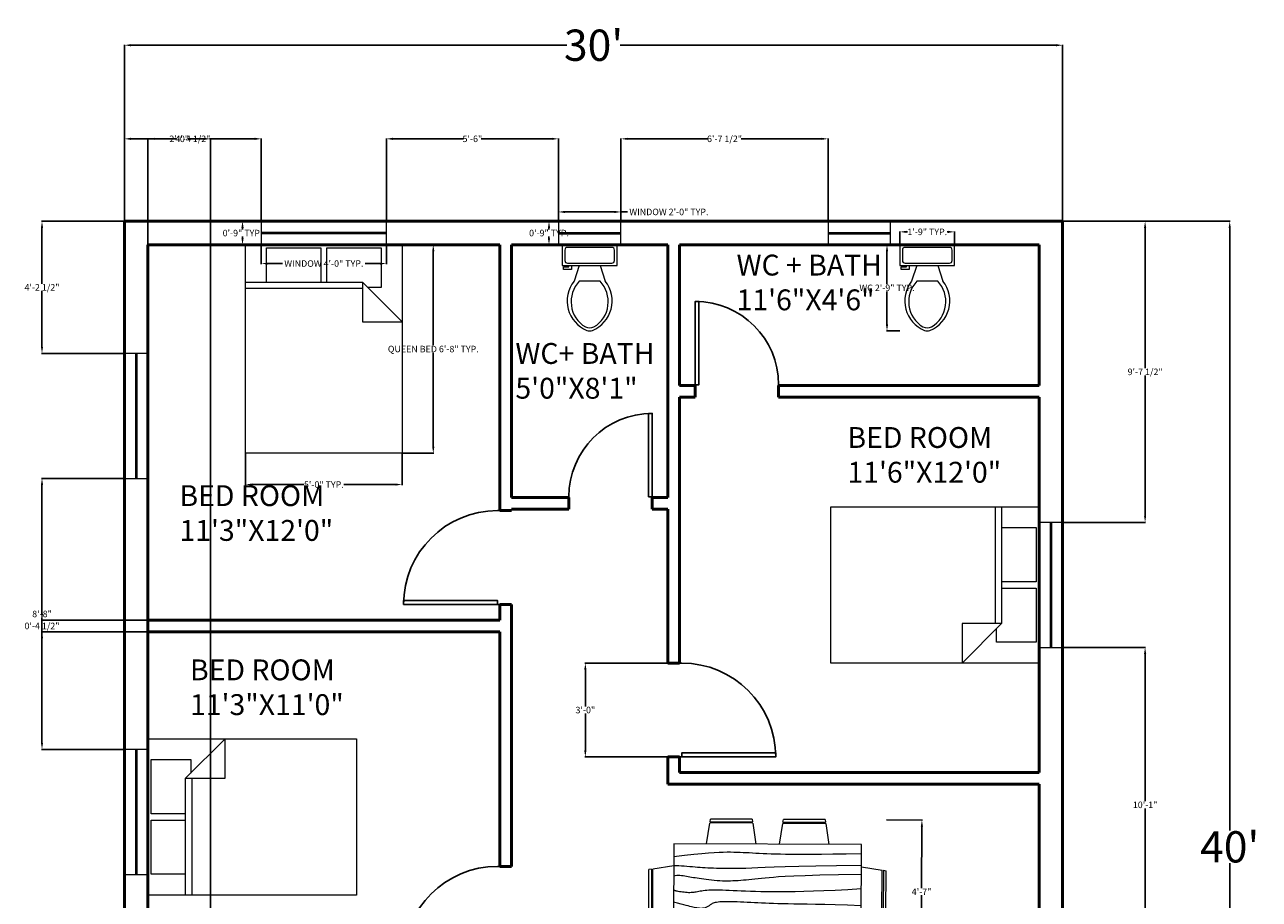
# Model space of a CAD drawing. Units: inches. Extents: x 14 to 510, y 5 to 635.
# Tile 3 of 3: x 18 to 492, y 299 to 635. Entities that reach past the tile are written whole.
import ezdxf

# ---------------------------------------------------------------- set-up
doc = ezdxf.new("R2010")
doc.units = ezdxf.units.IN
doc.header["$MEASUREMENT"] = 0
for name, color, linetype, lineweight in [('A-ANNO-DIMS', 210, 'Continuous', 18), ('A-AREA-IDEN', 210, 'Continuous', 25), ('A-FLOR-FIXT', 100, 'Continuous', 18), ('A-FURN', 100, 'Continuous', 18), ('DOOR', 20, 'Continuous', 25), ('WALL', 40, 'Continuous', 50), ('WINDOW', 131, 'Continuous', 18)]:
    doc.layers.add(name, color=color, linetype=linetype, lineweight=lineweight)
doc.styles.get("Standard").update_dxf_attribs({"font": 'arial.ttf'})
doc.dimstyles.get("Standard").update_dxf_attribs({"dimtxt": 2.5, "dimasz": 2.5, "dimexe": 0.18, "dimexo": 0.0625, "dimgap": 0.09, "dimtad": 0, "dimtih": 1, "dimtoh": 1, "dimzin": 0, "dimdsep": 46, "dimlunit": 3, "dimtxsty": 'Standard', "dimcen": 0.09, "dimadec": 0, "dimazin": 0, "dimtfac": 1, "dimtofl": 0, "dimtmove": 0, "dimatfit": 3, "dimfxl": 1, "dimtolj": 1, "dimtzin": 0, "dimarcsym": 0})

# ---------------------------------------------------------------- blocks, each defined once
blk = doc.blocks.new('*U2')
for p, q in [((0, 0), (0, -6)), ((40, 0), (40, -6))]:
    blk.add_line(p, q)
blk.add_lwpolyline([(0, 0), (0, 40), (1.75, 40), (1.75, 0)], close=True)
blk.add_arc((0, 0), 40, 0, 90)
blk = doc.blocks.new('Dining Set - 36 x 72 in.')
for p, q in [((-22.2343, 26.00059), (-23.4847, 17.99762)), ((-22.2304, 26), (-5.7608, 26)), ((-22, 27.5), (-22.1562, 26.50042)), ((-5.8416, 26.5), (-22.1534, 26.5)), ((-22, 27.5), (-6, 27.5)), ((-5.8437, 26.49966), (-6, 27.5)), ((-4.5152, 17.99762), (-5.7655, 25.99926)), ((5.7657, 26.00059), (4.5153, 17.99762)), ((5.7696, 26), (22.2392, 26)), ((6, 27.5), (5.8438, 26.50042)), ((22.1584, 26.5), (5.8466, 26.5)), ((6, 27.5), (22, 27.5)), ((22.1563, 26.49966), (22, 27.5)), ((23.4848, 17.99762), (22.2345, 25.99926)), ((36, 18), (-36, 18)), ((-36, 18), (-36, -18)), ((36, -18), (36, 18)), ((-44.0006, 8.23428), (-35.9976, 9.48474)), ((44.0006, 8.23428), (35.9976, 9.48474)), ((-45.5, 8), (-44.5004, 8.15617)), ((-45.5, 8), (-45.5, -8)), ((-44.5, -8.15843), (-44.5, 8.15338)), ((-44, 8.23041), (-44, -8.23915)), ((44, 8.23041), (44, -8.23915)), ((44.5, -8.15843), (44.5, 8.15338)), ((45.5, 8), (44.5005, 8.15617)), ((45.5, 8), (45.5, -8)), ((-44.4997, -8.15631), (-45.5, -8)), ((-35.9976, -9.48476), (-43.9993, -8.2345)), ((35.9976, -9.48476), (43.9993, -8.2345)), ((44.4997, -8.15631), (45.5, -8)), ((-36, -18), (36, -18)), ((-22.2343, -26.0006), (-23.4847, -17.99762)), ((-4.5152, -17.99762), (-5.7655, -25.99928)), ((5.7657, -26.0006), (4.5153, -17.99762)), ((23.4848, -17.99762), (22.2345, -25.99928)), ((-22.2304, -26), (-5.7608, -26)), ((-22, -27.5), (-22.1562, -26.50044)), ((-5.8416, -26.5), (-22.1534, -26.5)), ((-22, -27.5), (-6, -27.5)), ((-5.8437, -26.49967), (-6, -27.5)), ((5.7696, -26), (22.2392, -26)), ((6, -27.5), (5.8438, -26.50044)), ((22.1584, -26.5), (5.8466, -26.5)), ((6, -27.5), (22, -27.5)), ((22.1563, -26.49967), (22, -27.5))]:
    blk.add_line(p, q)
for points in [[(-36, 15), (-31.1772, 14.97754), (-26.8079, 14.91406), (-22.8538, 14.81543), (-19.276, 14.6875), (-16.0362, 14.53613), (-13.0957, 14.36718), (-10.4159, 14.18652), (-7.9583, 14), (-5.6904, 13.81315), (-3.6035, 13.63021), (-1.6954, 13.45508), (0.0365, 13.29166), (1.5945, 13.14388), (2.9811, 13.01562), (4.1988, 12.9108), (5.25, 12.83333), (6.1393, 12.78613), (6.8802, 12.76823), (7.4883, 12.77767), (7.9792, 12.8125), (8.3685, 12.87077), (8.6719, 12.95052), (8.9049, 13.0498), (9.0833, 13.16666), (9.2205, 13.29899), (9.3216, 13.44401), (9.3895, 13.59879), (9.4271, 13.76041), (9.4373, 13.92594), (9.4232, 14.09245), (9.3875, 14.257), (9.3333, 14.41666), (9.2638, 14.56917), (9.1836, 14.71484), (9.0975, 14.85465), (9.0104, 14.98958), (8.9272, 15.1206), (8.8529, 15.2487), (8.7922, 15.37483), (8.75, 15.5), (8.7305, 15.62467), (8.7344, 15.74739), (8.7617, 15.86621), (8.8125, 15.97916), (8.8867, 16.08431), (8.9844, 16.17968), (9.1055, 16.26334), (9.25, 16.33333), (9.4189, 16.38802), (9.6172, 16.42708), (9.8506, 16.45052), (10.125, 16.45833), (10.4463, 16.45052), (10.8203, 16.42708), (11.2529, 16.38802), (11.75, 16.33333), (12.3184, 16.26318), (12.9694, 16.17838), (13.7151, 16.07991), (14.5677, 15.96875), (15.5395, 15.84586), (16.6426, 15.71224), (17.8893, 15.56884), (19.2917, 15.41666), (20.859, 15.25667), (22.5879, 15.08984), (24.4721, 14.91715), (26.5052, 14.73958), (28.6809, 14.5581), (30.9929, 14.3737), (33.4347, 14.18733), (36, 14)], [(-36, 10), (-28.9766, 10.14274), (-23.1725, 10.20442), (-18.4241, 10.19775), (-14.5677, 10.13541), (-11.4399, 10.03011), (-8.877, 9.89453), (-6.7154, 9.74137), (-4.7917, 9.58333), (-2.9698, 9.43082), (-1.2246, 9.28515), (0.4415, 9.14534), (2.026, 9.01041), (3.5266, 8.87939), (4.9408, 8.7513), (6.266, 8.62516), (7.5, 8.5), (8.6411, 8.37549), (9.6914, 8.2539), (10.6538, 8.13818), (11.5312, 8.03125), (12.3267, 7.93603), (13.043, 7.85547), (13.6831, 7.79248), (14.25, 7.75), (14.7471, 7.7303), (15.1797, 7.73307), (15.5537, 7.75732), (15.875, 7.80208), (16.1494, 7.86637), (16.3828, 7.94922), (16.5811, 8.04964), (16.75, 8.16666), (16.8944, 8.29915), (17.0143, 8.44531), (17.1089, 8.60319), (17.1771, 8.77083), (17.218, 8.94629), (17.2305, 9.1276), (17.2137, 9.31282), (17.1667, 9.5), (17.0895, 9.6875), (16.987, 9.875), (16.8649, 10.0625), (16.7292, 10.25), (16.5856, 10.4375), (16.4401, 10.625), (16.2985, 10.8125), (16.1667, 11), (16.05, 11.18733), (15.9518, 11.3737), (15.8752, 11.5581), (15.8229, 11.73958), (15.798, 11.91715), (15.8034, 12.08984), (15.842, 12.25667), (15.9167, 12.41666), (16.0295, 12.56836), (16.1784, 12.70833), (16.3605, 12.83268), (16.5729, 12.9375), (16.8127, 13.01888), (17.0768, 13.07291), (17.3625, 13.0957), (17.6667, 13.08333), (17.9894, 13.03312), (18.3418, 12.94726), (18.7382, 12.82918), (19.1927, 12.68229), (19.7195, 12.51001), (20.3327, 12.31575), (21.0465, 12.10294), (21.875, 11.875), (22.8357, 11.63354), (23.959, 11.37304), (25.2786, 11.08618), (26.8282, 10.76562), (28.6414, 10.40405), (30.752, 9.99414), (33.1936, 9.52856), (36, 9)], [(-36, 5.5), (-30.7157, 5.3348), (-26.069, 5.20963), (-21.9946, 5.11767), (-18.4271, 5.05208), (-15.3009, 5.00602), (-12.5508, 4.97265), (-10.1112, 4.94515), (-7.9167, 4.91666), (-5.909, 4.88167), (-4.0586, 4.83984), (-2.3429, 4.79215), (-0.7396, 4.73958), (0.7739, 4.6831), (2.22, 4.6237), (3.6213, 4.56233), (5, 4.5), (6.373, 4.43782), (7.7344, 4.3776), (9.0723, 4.32129), (10.375, 4.27083), (11.6309, 4.22819), (12.8281, 4.19531), (13.9551, 4.17415), (15, 4.16666), (15.954, 4.17448), (16.819, 4.19791), (17.6001, 4.23698), (18.3021, 4.29166), (18.9299, 4.36198), (19.4883, 4.44791), (19.9823, 4.54948), (20.4167, 4.66666), (20.7969, 4.79899), (21.1302, 4.94401), (21.4245, 5.09879), (21.6875, 5.26041), (21.9271, 5.42594), (22.1511, 5.59245), (22.3672, 5.757), (22.5834, 5.91666), (22.8065, 6.06868), (23.0404, 6.21093), (23.2879, 6.34147), (23.5521, 6.45833), (23.8358, 6.55957), (24.142, 6.64323), (24.4735, 6.70735), (24.8334, 6.75), (25.2235, 6.76969), (25.642, 6.76692), (26.0858, 6.74267), (26.5521, 6.69791), (27.0379, 6.63362), (27.5404, 6.55078), (28.0565, 6.45036), (28.5834, 6.33333), (29.1242, 6.19987), (29.7071, 6.04687), (30.3661, 5.87044), (31.1354, 5.66666), (32.0493, 5.43164), (33.142, 5.16146), (34.4475, 4.85221), (36, 4.5)], [(-36, -1), (-30.7915, -0.6591), (-26.0195, -0.38216), (-21.6519, -0.16284), (-17.6563, 0.00521), (-14.0005, 0.12833), (-10.6523, 0.21289), (-7.5796, 0.26522), (-4.75, 0.29166), (-2.134, 0.29793), (0.2878, 0.28711), (2.5317, 0.26163), (4.6146, 0.22396), (6.5529, 0.17651), (8.3633, 0.12174), (10.0623, 0.06209), (11.6667, 0), (13.1899, -0.06201), (14.6341, -0.1211), (15.9982, -0.17432), (17.2813, -0.21875), (18.4823, -0.25147), (19.6003, -0.26953), (20.6343, -0.27002), (21.5834, -0.25), (22.4481, -0.20768), (23.2357, -0.14584), (23.9549, -0.06836), (24.6146, 0.02083), (25.2235, 0.11784), (25.7904, 0.21875), (26.3241, 0.31966), (26.8334, 0.41666), (27.3265, 0.50618), (27.8099, 0.58593), (28.2894, 0.65397), (28.7709, 0.70833), (29.2601, 0.74707), (29.763, 0.76823), (30.2855, 0.76985), (30.8334, 0.75), (31.4088, 0.70784), (31.9994, 0.64713), (32.589, 0.57275), (33.1615, 0.48958), (33.7008, 0.4025), (34.1908, 0.3164), (34.6153, 0.23616), (34.9584, 0.16666), (35.2099, 0.11165), (35.3848, 0.07031), (35.504, 0.04069), (35.5886, 0.02083), (35.6594, 0.00879), (35.7377, 0.0026), (35.8442, 0.00032), (36, 0)], [(-36, -6.5), (-27.1843, -6.31267), (-20.084, -6.1263), (-14.469, -5.9419), (-10.1094, -5.76042), (-6.7752, -5.58285), (-4.2363, -5.41016), (-2.2629, -5.24333), (-0.625, -5.08334), (0.8708, -4.93099), (2.2715, -4.78646), (3.5872, -4.64974), (4.8281, -4.52084), (6.0046, -4.39974), (7.127, -4.28646), (8.2053, -4.18099), (9.25, -4.08334), (10.2705, -3.99382), (11.2734, -3.91407), (12.2647, -3.84603), (13.25, -3.79167), (14.2354, -3.75293), (15.2266, -3.73177), (16.2295, -3.73015), (17.25, -3.75), (18.2912, -3.79248), (19.3451, -3.85547), (20.4009, -3.93604), (21.4479, -4.03125), (22.4754, -4.13819), (23.4727, -4.25391), (24.4289, -4.37549), (25.3334, -4.5), (26.1785, -4.62492), (26.9694, -4.74935), (27.7145, -4.87281), (28.4219, -4.99479), (29.1, -5.11483), (29.7572, -5.23242), (30.4016, -5.34709), (31.0417, -5.45834), (31.6837, -5.56437), (32.3262, -5.65821), (32.9658, -5.73153), (33.599, -5.77604), (34.2224, -5.78345), (34.8327, -5.74545), (35.4264, -5.65373), (36, -5.5)], [(-36, -10), (-26.4022, -9.81299), (-18.4675, -9.62891), (-11.9839, -9.45069), (-6.7396, -9.28125), (-2.5226, -9.12354), (0.8789, -8.98047), (3.6769, -8.85498), (6.0833, -8.75), (8.2767, -8.66765), (10.3021, -8.60677), (12.1712, -8.56543), (13.8958, -8.54167), (15.4876, -8.53353), (16.9583, -8.53907), (18.3197, -8.55632), (19.5834, -8.58334), (20.7616, -8.61841), (21.8685, -8.66081), (22.9188, -8.71004), (23.9271, -8.76563), (24.9081, -8.82707), (25.8763, -8.89388), (26.8465, -8.96558), (27.8334, -9.04167), (28.8474, -9.12118), (29.8828, -9.20117), (30.93, -9.27824), (31.9792, -9.34896), (33.0205, -9.40991), (34.0443, -9.45768), (35.0407, -9.48885), (36, -9.5)], [(-36, -14.5), (-30.0881, -14.33513), (-25.0332, -14.21224), (-20.7312, -14.12647), (-17.0781, -14.07292), (-13.97, -14.04671), (-11.3027, -14.04297), (-8.9724, -14.05681), (-6.875, -14.08334), (-4.9224, -14.11833), (-3.0905, -14.16016), (-1.3709, -14.20785), (0.2448, -14.26042), (1.7647, -14.3169), (3.1973, -14.3763), (4.5507, -14.43767), (5.8333, -14.5), (7.0554, -14.5621), (8.235, -14.62175), (9.3922, -14.67652), (10.5469, -14.72396), (11.7192, -14.76164), (12.929, -14.78711), (14.1965, -14.79794), (15.5417, -14.79167), (16.9933, -14.76424), (18.6152, -14.70508), (20.4804, -14.60197), (22.6615, -14.44271), (25.2312, -14.21509), (28.2624, -13.9069), (31.8277, -13.50594), (36, -13)]]:
    blk.add_lwpolyline(points)
blk = doc.blocks.new('Bed - Queen')
for p, q in [((0, -80.00003), (0, 0)), ((0, 0), (59.99999, 0)), ((59.99999, 0), (59.99999, -80.00003)), ((7.99999, -1.2), (28.79998, -1.2)), ((7.99999, -14.4), (7.99999, -1.2)), ((28.79998, -1.2), (28.79998, -14.4)), ((31.19999, -1.2), (51.99999, -1.2)), ((31.19999, -14.4), (31.19999, -1.2)), ((51.99999, -1.2), (51.99999, -16.4)), ((0, -14.4), (44.8, -14.4)), ((44.8, -16.8), (0, -16.8)), ((59.99999, -29.6), (44.8, -14.4)), ((44.8, -14.4), (44.8, -29.6)), ((51.99999, -16.4), (46.79936, -16.4)), ((44.8, -29.6), (59.99999, -29.6)), ((59.99999, -80.00003), (0, -80.00003))]:
    blk.add_line(p, q)
blk = doc.blocks.new('Toilet - top')
for p, q in [((9.5, -6), (9.5, -2)), ((-10, -8.5), (-8, -8.5)), ((-10, -9.5), (-10, -8.5)), ((-8, -8.5), (-8, -8)), ((-7, -8), (-7, -9.5)), ((-4, -8), (-6, -14)), ((4, -8), (6, -14)), ((-7, -9.5), (-10, -9.5)), ((4, -14), (-4, -14))]:
    blk.add_line(p, q)
blk.add_lwpolyline([(10.5, -8), (10.5, 0), (-10.5, 0), (-10.5, -8)], close=True)
for points in [[(-9.5, -2), (-9.5, -6)], [(8.5, -1), (-8.5, -1)], [(-8.5, -7), (8.5, -7)]]:
    blk.add_lwpolyline(points)
for centre, radius, start, end in [((-8.62, -1.88), 0.884, 81.8699, 188.1301), ((8.62, -1.88), 0.884, 351.8699, 98.1301), ((-8.62, -6.12), 0.884, 171.8699, 278.1301), ((8.62, -6.12), 0.884, 261.8699, 8.1301), ((3.52, -21.58), 12.17, 141.4691, 247.9714), ((4.2, -21.82), 11.33, 136.3677, 238.9468), ((-3.52, -21.58), 12.17, 292.0284, 38.5307), ((-4.2, -21.82), 11.33, 301.053, 43.6321), ((0, -27.88), 4, 245.7318, 294.2682), ((0, -29), 4, 254.8605, 285.1395)]:
    blk.add_arc(centre, radius, start, end)
blk = doc.blocks.new('*D14')
at = {"layer": 'A-ANNO-DIMS', "color": 0, "lineweight": -2, "transparency": 16777216}
for p, q in [((416.67, 559.06), (480.9, 559.06)), ((480.72, 556.56), (480.72, 325.28)), ((480.72, 81.56), (480.72, 312.84)), ((416.67, 79.06), (480.9, 79.06))]:
    blk.add_line(p, q, dxfattribs=at)
at = {"layer": 'A-ANNO-DIMS', "color": 0, "transparency": 16777216}
for points in [[(480.3, 556.56), (481.13, 556.56), (480.72, 559.06)], [(480.3, 81.56), (481.13, 81.56), (480.72, 79.06)]]:
    blk.add_solid(points, dxfattribs=at)
at = {"layer": 'Defpoints', "color": 0, "transparency": 16777216}
for p in [(416.61, 559.06), (416.61, 79.06), (480.72, 79.06)]:
    blk.add_point(p, dxfattribs=at)
at = {"layer": 'A-ANNO-DIMS', "color": 0, "transparency": 16777216, "insert": (480.72, 319.06), "char_height": 12, "attachment_point": 5}
blk.add_mtext("\\A1;40'", dxfattribs=at)
blk = doc.blocks.new('*D15')
at = {"layer": 'A-ANNO-DIMS', "color": 0, "lineweight": -2, "transparency": 16777216}
for p, q in [((56.61, 559.12), (56.61, 626.81)), ((59.11, 626.63), (226.34, 626.63)), ((414.11, 626.63), (246.88, 626.63)), ((416.61, 559.12), (416.61, 626.81))]:
    blk.add_line(p, q, dxfattribs=at)
at = {"layer": 'A-ANNO-DIMS', "color": 0, "transparency": 16777216}
for points in [[(59.11, 627.05), (59.11, 626.21), (56.61, 626.63)], [(414.11, 627.05), (414.11, 626.21), (416.61, 626.63)]]:
    blk.add_solid(points, dxfattribs=at)
at = {"layer": 'Defpoints', "color": 0, "transparency": 16777216}
for p in [(416.61, 626.63), (56.61, 559.06), (416.61, 559.06)]:
    blk.add_point(p, dxfattribs=at)
at = {"layer": 'A-ANNO-DIMS', "color": 0, "transparency": 16777216, "insert": (236.61, 626.63), "char_height": 12, "attachment_point": 5}
blk.add_mtext("\\A1;30'", dxfattribs=at)
blk = doc.blocks.new('WIN-48IN')
for p, q in [((4.25, 48), (4.25, 0)), ((4.75, 48), (4.75, 0))]:
    blk.add_line(p, q)
blk.add_lwpolyline([(0, 48), (0, 0), (9, 0), (9, 48)], close=True)
blk = doc.blocks.new('WIN-24IN')
for p, q in [((0, 4.75), (24, 4.75)), ((0, 4.25), (24, 4.25))]:
    blk.add_line(p, q)
blk.add_lwpolyline([(0, 0), (24, 0), (24, 9), (0, 9)], close=True)
blk = doc.blocks.new('*D19')
at = {"layer": 'A-ANNO-DIMS', "color": 0, "lineweight": -2, "transparency": 16777216}
for p, q in [((109.11, 550), (109.11, 542.68)), ((157.11, 550), (157.11, 542.68)), ((111.61, 542.86), (117.2, 542.86)), ((154.61, 542.86), (149.02, 542.86))]:
    blk.add_line(p, q, dxfattribs=at)
at = {"layer": 'A-ANNO-DIMS', "color": 0, "transparency": 16777216}
for points in [[(111.61, 543.28), (111.61, 542.44), (109.11, 542.86)], [(154.61, 543.28), (154.61, 542.44), (157.11, 542.86)]]:
    blk.add_solid(points, dxfattribs=at)
at = {"layer": 'Defpoints', "color": 0, "transparency": 16777216}
for p in [(109.11, 550.06), (157.11, 550.06), (157.11, 542.86)]:
    blk.add_point(p, dxfattribs=at)
at = {"layer": 'A-ANNO-DIMS', "color": 0, "transparency": 16777216, "insert": (133.11, 542.86), "char_height": 2.5, "attachment_point": 5}
blk.add_mtext('\\A1;WINDOW 4\'-0" TYP.', dxfattribs=at)
blk = doc.blocks.new('*D20')
at = {"layer": 'A-ANNO-DIMS', "color": 0, "lineweight": -2, "transparency": 16777216}
for p, q in [((109.05, 559.06), (101.73, 559.06)), ((101.91, 556.56), (101.91, 555.93)), ((109.05, 550.06), (101.73, 550.06)), ((101.91, 552.56), (101.91, 553.19))]:
    blk.add_line(p, q, dxfattribs=at)
at = {"layer": 'A-ANNO-DIMS', "color": 0, "transparency": 16777216}
for points in [[(101.49, 556.56), (102.33, 556.56), (101.91, 559.06)], [(101.49, 552.56), (102.33, 552.56), (101.91, 550.06)]]:
    blk.add_solid(points, dxfattribs=at)
at = {"layer": 'Defpoints', "color": 0, "transparency": 16777216}
for p in [(109.11, 559.06), (101.91, 550.06), (109.11, 550.06)]:
    blk.add_point(p, dxfattribs=at)
at = {"layer": 'A-ANNO-DIMS', "color": 0, "transparency": 16777216, "insert": (101.91, 554.56), "char_height": 2.5, "attachment_point": 5}
blk.add_mtext('\\A1;0\'-9" TYP.', dxfattribs=at)
blk = doc.blocks.new('*D23')
at = {"layer": 'A-ANNO-DIMS', "color": 0, "lineweight": -2, "transparency": 16777216}
for p, q in [((223.11, 559.12), (223.11, 562.84)), ((225.61, 562.66), (244.61, 562.66)), ((247.11, 559.12), (247.11, 562.84)), ((247.11, 562.66), (249.61, 562.66))]:
    blk.add_line(p, q, dxfattribs=at)
at = {"layer": 'A-ANNO-DIMS', "color": 0, "transparency": 16777216}
for points in [[(225.61, 563.08), (225.61, 562.24), (223.11, 562.66)], [(244.61, 563.08), (244.61, 562.24), (247.11, 562.66)]]:
    blk.add_solid(points, dxfattribs=at)
at = {"layer": 'Defpoints', "color": 0, "transparency": 16777216}
for p in [(223.11, 559.06), (247.11, 562.66), (247.11, 559.06)]:
    blk.add_point(p, dxfattribs=at)
at = {"layer": 'A-ANNO-DIMS', "color": 0, "transparency": 16777216, "insert": (265.52, 562.66), "char_height": 2.5, "attachment_point": 5}
blk.add_mtext('\\A1;WINDOW 2\'-0" TYP.', dxfattribs=at)
blk = doc.blocks.new('*D24')
at = {"layer": 'A-ANNO-DIMS', "color": 0, "lineweight": -2, "transparency": 16777216}
for p, q in [((223.05, 559.06), (219.33, 559.06)), ((219.51, 556.56), (219.51, 555.93)), ((223.05, 550.06), (219.33, 550.06)), ((219.51, 552.56), (219.51, 553.19))]:
    blk.add_line(p, q, dxfattribs=at)
at = {"layer": 'A-ANNO-DIMS', "color": 0, "transparency": 16777216}
for points in [[(219.09, 556.56), (219.93, 556.56), (219.51, 559.06)], [(219.09, 552.56), (219.93, 552.56), (219.51, 550.06)]]:
    blk.add_solid(points, dxfattribs=at)
at = {"layer": 'Defpoints', "color": 0, "transparency": 16777216}
for p in [(219.51, 559.06), (223.11, 559.06), (223.11, 550.06)]:
    blk.add_point(p, dxfattribs=at)
at = {"layer": 'A-ANNO-DIMS', "color": 0, "transparency": 16777216, "insert": (219.51, 554.56), "char_height": 2.5, "attachment_point": 5}
blk.add_mtext('\\A1;0\'-9" TYP.', dxfattribs=at)
blk = doc.blocks.new('*D25')
at = {"layer": 'A-ANNO-DIMS', "color": 0, "lineweight": -2, "transparency": 16777216}
for p, q in [((163.17, 550.06), (175.29, 550.06)), ((175.11, 547.56), (175.11, 511.52)), ((175.11, 472.56), (175.11, 508.6)), ((163.17, 470.06), (175.29, 470.06))]:
    blk.add_line(p, q, dxfattribs=at)
at = {"layer": 'A-ANNO-DIMS', "color": 0, "transparency": 16777216}
for points in [[(174.69, 547.56), (175.53, 547.56), (175.11, 550.06)], [(174.69, 472.56), (175.53, 472.56), (175.11, 470.06)]]:
    blk.add_solid(points, dxfattribs=at)
at = {"layer": 'Defpoints', "color": 0, "transparency": 16777216}
for p in [(163.11, 550.06), (175.11, 550.06), (163.11, 470.06)]:
    blk.add_point(p, dxfattribs=at)
at = {"layer": 'A-ANNO-DIMS', "color": 0, "transparency": 16777216, "insert": (175.11, 510.06), "char_height": 2.5, "attachment_point": 5}
blk.add_mtext('\\A1;QUEEN BED 6\'-8" TYP.', dxfattribs=at)
blk = doc.blocks.new('*D26')
at = {"layer": 'A-ANNO-DIMS', "color": 0, "lineweight": -2, "transparency": 16777216}
for p, q in [((103.11, 470), (103.11, 457.88)), ((163.11, 470), (163.11, 457.88)), ((105.61, 458.06), (125.4, 458.06)), ((160.61, 458.06), (140.82, 458.06))]:
    blk.add_line(p, q, dxfattribs=at)
at = {"layer": 'A-ANNO-DIMS', "color": 0, "transparency": 16777216}
for points in [[(105.61, 458.48), (105.61, 457.64), (103.11, 458.06)], [(160.61, 458.48), (160.61, 457.64), (163.11, 458.06)]]:
    blk.add_solid(points, dxfattribs=at)
at = {"layer": 'Defpoints', "color": 0, "transparency": 16777216}
for p in [(103.11, 470.06), (163.11, 470.06), (163.11, 458.06)]:
    blk.add_point(p, dxfattribs=at)
at = {"layer": 'A-ANNO-DIMS', "color": 0, "transparency": 16777216, "insert": (133.11, 458.06), "char_height": 2.5, "attachment_point": 5}
blk.add_mtext('\\A1;5\'-0" TYP.', dxfattribs=at)
blk = doc.blocks.new('*D27')
at = {"layer": 'A-ANNO-DIMS', "color": 0, "lineweight": -2, "transparency": 16777216}
for p, q in [((354.1, 550.06), (349.03, 550.06)), ((349.21, 547.56), (349.21, 534.92)), ((349.21, 519.51), (349.21, 532.16)), ((354.1, 517.01), (349.03, 517.01))]:
    blk.add_line(p, q, dxfattribs=at)
at = {"layer": 'A-ANNO-DIMS', "color": 0, "transparency": 16777216}
for points in [[(348.79, 547.56), (349.63, 547.56), (349.21, 550.06)], [(348.79, 519.51), (349.63, 519.51), (349.21, 517.01)]]:
    blk.add_solid(points, dxfattribs=at)
at = {"layer": 'Defpoints', "color": 0, "transparency": 16777216}
for p in [(349.21, 550.06), (354.17, 550.06), (354.17, 517.01)]:
    blk.add_point(p, dxfattribs=at)
at = {"layer": 'A-ANNO-DIMS', "color": 0, "transparency": 16777216, "insert": (349.21, 533.54), "char_height": 2.5, "attachment_point": 5}
blk.add_mtext('\\A1;WC 2\'-9" TYP.', dxfattribs=at)
blk = doc.blocks.new('*D28')
at = {"layer": 'A-ANNO-DIMS', "color": 0, "lineweight": -2, "transparency": 16777216}
for p, q in [((354.17, 550.12), (354.17, 555.2)), ((356.67, 555.02), (357.07, 555.02)), ((372.67, 555.02), (372.26, 555.02)), ((375.17, 550.12), (375.17, 555.2))]:
    blk.add_line(p, q, dxfattribs=at)
at = {"layer": 'A-ANNO-DIMS', "color": 0, "transparency": 16777216}
for points in [[(356.67, 555.43), (356.67, 554.6), (354.17, 555.02)], [(372.67, 555.43), (372.67, 554.6), (375.17, 555.02)]]:
    blk.add_solid(points, dxfattribs=at)
at = {"layer": 'Defpoints', "color": 0, "transparency": 16777216}
for p in [(375.17, 555.02), (354.17, 550.06), (375.17, 550.06)]:
    blk.add_point(p, dxfattribs=at)
at = {"layer": 'A-ANNO-DIMS', "color": 0, "transparency": 16777216, "insert": (364.67, 555.02), "char_height": 2.5, "attachment_point": 5}
blk.add_mtext('\\A1;1\'-9" TYP.', dxfattribs=at)
blk = doc.blocks.new('*D30')
at = {"layer": 'A-ANNO-DIMS', "color": 0, "lineweight": -2, "transparency": 16777216}
for p, q in [((349.02, 329.39), (362.79, 329.33)), ((362.6, 326.83), (362.49, 303.17)), ((362.36, 276.83), (362.47, 300.49)), ((348.76, 274.39), (362.53, 274.33))]:
    blk.add_line(p, q, dxfattribs=at)
at = {"layer": 'A-ANNO-DIMS', "color": 0, "transparency": 16777216}
for points in [[(362.18, 326.83), (363.02, 326.82), (362.61, 329.33)], [(361.95, 276.83), (362.78, 276.83), (362.35, 274.33)]]:
    blk.add_solid(points, dxfattribs=at)
at = {"layer": 'Defpoints', "color": 0, "transparency": 16777216}
for p in [(348.96, 329.39), (348.7, 274.39), (362.35, 274.33)]:
    blk.add_point(p, dxfattribs=at)
at = {"layer": 'A-ANNO-DIMS', "color": 0, "transparency": 16777216, "insert": (362.48, 301.83), "char_height": 2.5, "attachment_point": 5}
blk.add_mtext('\\A1;4\'-7"', dxfattribs=at)
blk = doc.blocks.new('*D39')
at = {"layer": 'A-ANNO-DIMS', "color": 0, "lineweight": -2, "transparency": 16777216}
for p, q in [((56.61, 559.12), (56.61, 590.89)), ((59.11, 590.71), (76.49, 590.71)), ((106.61, 590.71), (89.24, 590.71)), ((109.11, 559.12), (109.11, 590.89))]:
    blk.add_line(p, q, dxfattribs=at)
at = {"layer": 'A-ANNO-DIMS', "color": 0, "transparency": 16777216}
for points in [[(59.11, 591.13), (59.11, 590.29), (56.61, 590.71)], [(106.61, 591.13), (106.61, 590.29), (109.11, 590.71)]]:
    blk.add_solid(points, dxfattribs=at)
at = {"layer": 'Defpoints', "color": 0, "transparency": 16777216}
for p in [(109.11, 590.71), (56.61, 559.06), (109.11, 559.06)]:
    blk.add_point(p, dxfattribs=at)
at = {"layer": 'A-ANNO-DIMS', "color": 0, "transparency": 16777216, "insert": (82.86, 590.71), "char_height": 2.5, "attachment_point": 5}
blk.add_mtext('\\A1;4\'-4 1/2"', dxfattribs=at)
blk = doc.blocks.new('*D40')
at = {"layer": 'A-ANNO-DIMS', "color": 0, "lineweight": -2, "transparency": 16777216}
for p, q in [((157.11, 559.12), (157.11, 590.89)), ((159.61, 590.71), (186.7, 590.71)), ((220.61, 590.71), (193.52, 590.71)), ((223.11, 559.12), (223.11, 590.89))]:
    blk.add_line(p, q, dxfattribs=at)
at = {"layer": 'A-ANNO-DIMS', "color": 0, "transparency": 16777216}
for points in [[(159.61, 591.13), (159.61, 590.29), (157.11, 590.71)], [(220.61, 591.13), (220.61, 590.29), (223.11, 590.71)]]:
    blk.add_solid(points, dxfattribs=at)
at = {"layer": 'Defpoints', "color": 0, "transparency": 16777216}
for p in [(223.11, 590.71), (157.11, 559.06), (223.11, 559.06)]:
    blk.add_point(p, dxfattribs=at)
at = {"layer": 'A-ANNO-DIMS', "color": 0, "transparency": 16777216, "insert": (190.11, 590.71), "char_height": 2.5, "attachment_point": 5}
blk.add_mtext('\\A1;5\'-6"', dxfattribs=at)
blk = doc.blocks.new('*D41')
at = {"layer": 'A-ANNO-DIMS', "color": 0, "lineweight": -2, "transparency": 16777216}
for p, q in [((247.11, 559.12), (247.11, 590.89)), ((249.61, 590.71), (280.53, 590.71)), ((324.11, 590.71), (293.19, 590.71)), ((326.61, 559.12), (326.61, 590.89))]:
    blk.add_line(p, q, dxfattribs=at)
at = {"layer": 'A-ANNO-DIMS', "color": 0, "transparency": 16777216}
for points in [[(249.61, 591.13), (249.61, 590.29), (247.11, 590.71)], [(324.11, 591.13), (324.11, 590.29), (326.61, 590.71)]]:
    blk.add_solid(points, dxfattribs=at)
at = {"layer": 'Defpoints', "color": 0, "transparency": 16777216}
for p in [(326.61, 590.71), (247.11, 559.06), (326.61, 559.06)]:
    blk.add_point(p, dxfattribs=at)
at = {"layer": 'A-ANNO-DIMS', "color": 0, "transparency": 16777216, "insert": (286.86, 590.71), "char_height": 2.5, "attachment_point": 5}
blk.add_mtext('\\A1;6\'-7 1/2"', dxfattribs=at)
blk = doc.blocks.new('*D46')
at = {"layer": 'A-ANNO-DIMS', "color": 0, "lineweight": -2, "transparency": 16777216}
for p, q in [((56.55, 559.06), (24.78, 559.06)), ((24.96, 556.56), (24.96, 535.11)), ((24.96, 510.89), (24.96, 532.34)), ((56.55, 508.39), (24.78, 508.39))]:
    blk.add_line(p, q, dxfattribs=at)
at = {"layer": 'A-ANNO-DIMS', "color": 0, "transparency": 16777216}
for points in [[(24.54, 556.56), (25.38, 556.56), (24.96, 559.06)], [(24.54, 510.89), (25.38, 510.89), (24.96, 508.39)]]:
    blk.add_solid(points, dxfattribs=at)
at = {"layer": 'Defpoints', "color": 0, "transparency": 16777216}
for p in [(56.61, 559.06), (24.96, 508.39), (56.61, 508.39)]:
    blk.add_point(p, dxfattribs=at)
at = {"layer": 'A-ANNO-DIMS', "color": 0, "transparency": 16777216, "insert": (24.96, 533.72), "char_height": 2.5, "attachment_point": 5}
blk.add_mtext('\\A1;4\'-2 1/2"', dxfattribs=at)
blk = doc.blocks.new('*D47')
at = {"layer": 'A-ANNO-DIMS', "color": 0, "lineweight": -2, "transparency": 16777216}
for p, q in [((56.55, 460.39), (24.78, 460.39)), ((24.96, 457.89), (24.96, 409.79)), ((24.96, 358.97), (24.96, 407.06)), ((56.55, 356.47), (24.78, 356.47))]:
    blk.add_line(p, q, dxfattribs=at)
at = {"layer": 'A-ANNO-DIMS', "color": 0, "transparency": 16777216}
for points in [[(24.54, 457.89), (25.38, 457.89), (24.96, 460.39)], [(24.54, 358.97), (25.38, 358.97), (24.96, 356.47)]]:
    blk.add_solid(points, dxfattribs=at)
at = {"layer": 'Defpoints', "color": 0, "transparency": 16777216}
for p in [(56.61, 460.39), (24.96, 356.47), (56.61, 356.47)]:
    blk.add_point(p, dxfattribs=at)
at = {"layer": 'A-ANNO-DIMS', "color": 0, "transparency": 16777216, "insert": (24.96, 408.43), "char_height": 2.5, "attachment_point": 5}
blk.add_mtext('\\A1;8\'-8"', dxfattribs=at)
blk = doc.blocks.new('*D48')
at = {"layer": 'A-ANNO-DIMS', "color": 0, "lineweight": -2, "transparency": 16777216}
for p, q in [((416.67, 559.06), (448.44, 559.06)), ((448.26, 556.56), (448.26, 502.69)), ((448.26, 446.06), (448.26, 499.93)), ((416.67, 443.56), (448.44, 443.56))]:
    blk.add_line(p, q, dxfattribs=at)
at = {"layer": 'A-ANNO-DIMS', "color": 0, "transparency": 16777216}
for points in [[(447.84, 556.56), (448.68, 556.56), (448.26, 559.06)], [(447.84, 446.06), (448.68, 446.06), (448.26, 443.56)]]:
    blk.add_solid(points, dxfattribs=at)
at = {"layer": 'Defpoints', "color": 0, "transparency": 16777216}
for p in [(416.61, 559.06), (416.61, 443.56), (448.26, 443.56)]:
    blk.add_point(p, dxfattribs=at)
at = {"layer": 'A-ANNO-DIMS', "color": 0, "transparency": 16777216, "insert": (448.26, 501.31), "char_height": 2.5, "attachment_point": 5}
blk.add_mtext('\\A1;9\'-7 1/2"', dxfattribs=at)
blk = doc.blocks.new('*D49')
at = {"layer": 'A-ANNO-DIMS', "color": 0, "lineweight": -2, "transparency": 16777216}
for p, q in [((416.67, 395.56), (448.44, 395.56)), ((448.26, 393.06), (448.26, 336.55)), ((448.26, 277.31), (448.26, 333.82)), ((416.67, 274.81), (448.44, 274.81))]:
    blk.add_line(p, q, dxfattribs=at)
at = {"layer": 'A-ANNO-DIMS', "color": 0, "transparency": 16777216}
for points in [[(447.84, 393.06), (448.68, 393.06), (448.26, 395.56)], [(447.84, 277.31), (448.68, 277.31), (448.26, 274.81)]]:
    blk.add_solid(points, dxfattribs=at)
at = {"layer": 'Defpoints', "color": 0, "transparency": 16777216}
for p in [(416.61, 395.56), (416.61, 274.81), (448.26, 274.81)]:
    blk.add_point(p, dxfattribs=at)
at = {"layer": 'A-ANNO-DIMS', "color": 0, "transparency": 16777216, "insert": (448.26, 335.19), "char_height": 2.5, "attachment_point": 5}
blk.add_mtext('\\A1;10\'-1"', dxfattribs=at)
blk = doc.blocks.new('*D52')
at = {"layer": 'A-ANNO-DIMS', "color": 0, "lineweight": -2, "transparency": 16777216}
for p, q in [((265.05, 389.56), (233.28, 389.56)), ((233.46, 387.06), (233.46, 372.93)), ((233.46, 356.06), (233.46, 370.19)), ((265.05, 353.56), (233.28, 353.56))]:
    blk.add_line(p, q, dxfattribs=at)
at = {"layer": 'A-ANNO-DIMS', "color": 0, "transparency": 16777216}
for points in [[(233.04, 387.06), (233.88, 387.06), (233.46, 389.56)], [(233.04, 356.06), (233.88, 356.06), (233.46, 353.56)]]:
    blk.add_solid(points, dxfattribs=at)
at = {"layer": 'Defpoints', "color": 0, "transparency": 16777216}
for p in [(233.46, 389.56), (265.11, 389.56), (265.11, 353.56)]:
    blk.add_point(p, dxfattribs=at)
at = {"layer": 'A-ANNO-DIMS', "color": 0, "transparency": 16777216, "insert": (233.46, 371.56), "char_height": 2.5, "attachment_point": 5}
blk.add_mtext('\\A1;3\'-0"', dxfattribs=at)
blk = doc.blocks.new('*D55')
at = {"layer": 'A-ANNO-DIMS', "color": 0, "lineweight": -2, "transparency": 16777216}
for p, q in [((24.96, 408.56), (24.96, 411.06)), ((65.55, 406.06), (24.78, 406.06)), ((65.55, 401.56), (24.78, 401.56)), ((24.96, 399.06), (24.96, 396.56))]:
    blk.add_line(p, q, dxfattribs=at)
at = {"layer": 'A-ANNO-DIMS', "color": 0, "transparency": 16777216}
for points in [[(24.54, 408.56), (25.38, 408.56), (24.96, 406.06)], [(24.54, 399.06), (25.38, 399.06), (24.96, 401.56)]]:
    blk.add_solid(points, dxfattribs=at)
at = {"layer": 'Defpoints', "color": 0, "transparency": 16777216}
for p in [(24.96, 406.06), (65.61, 406.06), (65.61, 401.56)]:
    blk.add_point(p, dxfattribs=at)
at = {"layer": 'A-ANNO-DIMS', "color": 0, "transparency": 16777216, "insert": (24.96, 403.81), "char_height": 2.5, "attachment_point": 5}
blk.add_mtext('\\A1;0\'-4 1/2"', dxfattribs=at)
blk = doc.blocks.new('*D56')
at = {"layer": 'A-ANNO-DIMS', "color": 0, "lineweight": -2, "transparency": 16777216}
for p, q in [((65.61, 182.62), (65.61, 590.89)), ((68.11, 590.71), (74.18, 590.71)), ((87.11, 590.71), (81.05, 590.71)), ((89.61, 182.62), (89.61, 590.89))]:
    blk.add_line(p, q, dxfattribs=at)
at = {"layer": 'A-ANNO-DIMS', "color": 0, "transparency": 16777216}
for points in [[(68.11, 591.13), (68.11, 590.29), (65.61, 590.71)], [(87.11, 591.13), (87.11, 590.29), (89.61, 590.71)]]:
    blk.add_solid(points, dxfattribs=at)
at = {"layer": 'Defpoints', "color": 0, "transparency": 16777216}
for p in [(89.61, 590.71), (65.61, 182.56), (89.61, 182.56)]:
    blk.add_point(p, dxfattribs=at)
at = {"layer": 'A-ANNO-DIMS', "color": 0, "transparency": 16777216, "insert": (77.61, 590.71), "char_height": 2.5, "attachment_point": 5}
blk.add_mtext('\\A1;2\'-0"', dxfattribs=at)

msp = doc.modelspace()

# ---------------------------------------------------------------- linework, layer by layer
at = {"layer": 'WALL'}
for p, q in [((65.611, 550.061), (65.611, 269.561)), ((200.611, 550.061), (65.611, 550.061)), ((200.611, 550.061), (200.611, 448.061)), ((205.111, 550.061), (205.111, 453.061)), ((265.111, 550.061), (205.111, 550.061)), ((265.111, 550.061), (265.111, 453.061)), ((407.611, 550.061), (269.611, 550.061)), ((269.611, 550.061), (269.611, 496.061)), ((407.611, 496.061), (407.611, 550.061)), ((275.611, 496.061), (269.611, 496.061)), ((275.611, 496.061), (275.611, 491.561)), ((407.611, 496.061), (307.611, 496.061)), ((307.611, 496.061), (307.611, 491.561)), ((275.611, 491.561), (269.611, 491.561)), ((269.611, 491.561), (269.611, 389.561)), ((407.611, 491.561), (307.611, 491.561)), ((407.611, 347.561), (407.611, 491.561)), ((227.111, 453.061), (205.111, 453.061)), ((227.111, 453.061), (227.111, 448.561)), ((265.111, 453.061), (259.111, 453.061)), ((259.111, 453.061), (259.111, 448.561)), ((200.611, 448.061), (205.111, 448.061)), ((227.111, 448.561), (205.111, 448.561)), ((205.111, 448.561), (205.111, 448.061)), ((265.111, 448.561), (259.111, 448.561)), ((265.111, 448.561), (265.111, 389.561)), ((200.611, 412.061), (205.111, 412.061)), ((200.611, 412.061), (200.611, 406.061)), ((205.111, 412.061), (205.111, 311.561)), ((200.611, 406.061), (65.611, 406.061)), ((200.611, 401.561), (65.611, 401.561)), ((200.611, 401.561), (200.611, 311.561)), ((269.611, 389.561), (265.111, 389.561)), ((269.611, 353.561), (265.111, 353.561)), ((265.111, 353.561), (265.111, 343.061)), ((269.611, 353.561), (269.611, 347.561)), ((407.611, 347.561), (269.611, 347.561)), ((407.611, 343.061), (265.111, 343.061)), ((407.611, 158.561), (407.611, 343.061)), ((200.611, 311.561), (205.111, 311.561))]:
    msp.add_line(p, q, dxfattribs=at)
msp.add_lwpolyline([(331.111, 79.061), (416.611, 79.061), (416.611, 559.061), (56.611, 559.061), (56.611, 79.061), (279.611, 79.061)], dxfattribs=at)
at = {"layer": 'WINDOW'}
for p, q in [((60.861, 508.387), (60.861, 460.387)), ((61.361, 508.387), (61.361, 460.387))]:
    msp.add_line(p, q, dxfattribs=at)
msp.add_lwpolyline([(56.611, 508.387), (56.611, 460.387), (65.611, 460.387), (65.611, 508.387)], close=True, dxfattribs=at)

# ---------------------------------------------------------------- block references
at = {"layer": 'A-FLOR-FIXT'}
for p in [(235.111, 550.061), (364.666, 550.061)]:
    msp.add_blockref('Toilet - top', p, dxfattribs=at)
at = {"layer": 'A-FURN'}
msp.add_blockref('Bed - Queen', (103.111, 550.061), dxfattribs=at)
for name, p, rotation in [('Bed - Queen', (407.611, 449.561), 270), ('Bed - Queen', (65.611, 300.551), 89.99999999999999), ('Dining Set - 36 x 72 in.', (303.331, 302.107), 179.7284420558059)]:
    msp.add_blockref(name, p, dxfattribs=dict(at, rotation=rotation))
at = {"layer": 'DOOR', "yscale": 0.8, "zscale": 0.8}
for p, xscale in [((275.611, 496.361), 0.8), ((259.111, 453.361), -0.8)]:
    msp.add_blockref('*U2', p, dxfattribs=dict(at, xscale=xscale))
at = {"layer": 'DOOR'}
for p, xscale, yscale, zscale, rotation in [((199.711, 412.061), 0.8999999999999971, 0.8999999999999971, 0.8999999999999971, 90), ((270.511, 353.561), -0.9, 0.9, 0.9, 270), ((199.711, 275.561), 0.9, 0.9, 0.9, 90)]:
    msp.add_blockref('*U2', p, dxfattribs=dict(at, xscale=xscale, yscale=yscale, zscale=zscale, rotation=rotation))
at = {"layer": 'WINDOW', "rotation": 270.0000000000005}
msp.add_blockref('WIN-48IN', (109.111, 559.061), dxfattribs=at)
at = {"layer": 'WINDOW'}
for name, p in [('WIN-24IN', (223.111, 550.061)), ('WIN-24IN', (326.611, 550.061)), ('WIN-48IN', (407.611, 395.561)), ('WIN-48IN', (56.611, 308.465))]:
    msp.add_blockref(name, p, dxfattribs=at)

# ---------------------------------------------------------------- texts
at = {"layer": 'A-AREA-IDEN', "char_height": 8, "attachment_point": 1}
for s, insert in [('WC + BATH\\P11\'6"X4\'6"', (291.491, 546.268)), ('WC+ BATH\\P5\'0"X8\'1"', (206.624, 512.36)), ('BED ROOM\\P11\'6"X12\'0"', (334.019, 480.12)), ('BED ROOM\\P11\'3"X12\'0"', (77.706, 457.803)), ('BED ROOM\\P11\'3"X11\'0"', (81.753, 390.966))]:
    msp.add_mtext_dynamic_manual_height_columns(s, width=74.81964, gutter_width=1, heights=[0], dxfattribs=dict(at, insert=insert))

# ---------------------------------------------------------------- dimensions: what is measured, and where the dimension line sits
at = {"layer": 'A-ANNO-DIMS'}
for p1, p2, distance, picture, middle in [((56.611, 559.061), (416.611, 559.061), 67.568, '*D15', (236.611, 626.629)), ((416.611, 559.061), (416.611, 79.061), 64.106, '*D14', (480.717, 319.061))]:
    dim = msp.add_aligned_dim(p1=p1, p2=p2, distance=distance, dimstyle='Standard', override={"dimtxt": 12, "dimclrd": 0, "dimclre": 0, "dimclrt": 0}, dxfattribs=at)
    dim.commit()
    dim.dimension.update_dxf_attribs({"geometry": picture, "text_midpoint": middle})
for base, p1, p2, picture, middle in [((109.111, 590.711), (56.611, 559.061), (109.111, 559.061), '*D39', (82.861, 590.711)), ((89.611, 590.711), (65.611, 182.561), (89.611, 182.561), '*D56', (77.611, 590.711)), ((223.111, 590.711), (157.111, 559.061), (223.111, 559.061), '*D40', (190.111, 590.711)), ((326.611, 590.711), (247.111, 559.061), (326.611, 559.061), '*D41', (286.861, 590.711))]:
    dim = msp.add_linear_dim(base=base, p1=p1, p2=p2, dimstyle='Standard', override={"dimdec": 1, "dimlfac": 1, "dimrnd": 0, "dimzin": 1, "dimdsep": 46, "dimlunit": 4, "dimfrac": 2}, dxfattribs=at)
    dim.commit()
    dim.dimension.update_dxf_attribs({"geometry": picture, "text_midpoint": middle})
for base, p1, p2, text, picture, middle in [((247.111, 562.661), (223.111, 559.061), (247.111, 559.061), 'WINDOW <> TYP.', '*D23', (265.519, 562.661)), ((375.166, 555.018), (354.166, 550.061), (375.166, 550.061), '<> TYP.', '*D28', (364.666, 555.018)), ((163.111, 458.061), (103.111, 470.061), (163.111, 470.061), '<> TYP.', '*D26', (133.111, 458.061))]:
    dim = msp.add_linear_dim(base=base, p1=p1, p2=p2, text=text, dimstyle='Standard', override={"dimdec": 1, "dimlfac": 1, "dimrnd": 0, "dimzin": 1, "dimdsep": 46, "dimlunit": 4, "dimfrac": 2}, dxfattribs=at)
    dim.commit()
    dim.dimension.update_dxf_attribs({"geometry": picture, "text_midpoint": middle})
for base, p1, p2, angle, picture, middle in [((24.961, 508.387), (56.611, 559.061), (56.611, 508.387), 90, '*D46', (24.961, 533.724)), ((448.261, 443.561), (416.611, 559.061), (416.611, 443.561), 90, '*D48', (448.261, 501.311)), ((24.961, 356.465), (56.611, 460.387), (56.611, 356.465), 90, '*D47', (24.961, 408.426)), ((24.961, 406.061), (65.611, 401.561), (65.611, 406.061), 90, '*D55', (24.961, 403.811)), ((448.260991, 274.811007), (416.610991, 395.561007), (416.610991, 274.811007), 90, '*D49', (448.260991, 335.186007)), ((233.461, 389.561), (265.111, 353.561), (265.111, 389.561), 90, '*D52', (233.461, 371.561)), ((362.35, 274.327), (348.961, 329.391), (348.7, 274.392), 269.72844, '*D30', (362.481, 301.827))]:
    dim = msp.add_linear_dim(base=base, p1=p1, p2=p2, angle=angle, dimstyle='Standard', override={"dimdec": 1, "dimlfac": 1, "dimrnd": 0, "dimzin": 1, "dimdsep": 46, "dimlunit": 4, "dimfrac": 2}, dxfattribs=at)
    dim.commit()
    dim.dimension.update_dxf_attribs({"geometry": picture, "text_midpoint": middle})
for base, p1, p2, angle, text, picture, middle in [((101.911, 550.061), (109.111, 559.061), (109.111, 550.061), 270, '<> TYP.', '*D20', (101.911, 554.561)), ((219.511, 559.061), (223.111, 550.061), (223.111, 559.061), 90, '<> TYP.', '*D24', (219.511, 554.561)), ((157.111, 542.861), (109.111, 550.061), (157.111, 550.061), 0, 'WINDOW <> TYP.', '*D19', (133.111, 542.861)), ((175.111, 550.061), (163.111, 470.061), (163.111, 550.061), 90, 'QUEEN BED <> TYP.', '*D25', (175.111, 510.061)), ((349.209, 550.061), (354.166, 517.015), (354.166, 550.061), 90, 'WC <> TYP.', '*D27', (349.209, 533.538))]:
    dim = msp.add_linear_dim(base=base, p1=p1, p2=p2, angle=angle, text=text, dimstyle='Standard', override={"dimdec": 1, "dimlfac": 1, "dimrnd": 0, "dimzin": 1, "dimdsep": 46, "dimlunit": 4, "dimfrac": 2}, dxfattribs=at)
    dim.commit()
    dim.dimension.update_dxf_attribs({"geometry": picture, "text_midpoint": middle})

doc.saveas('drawing.dxf')
